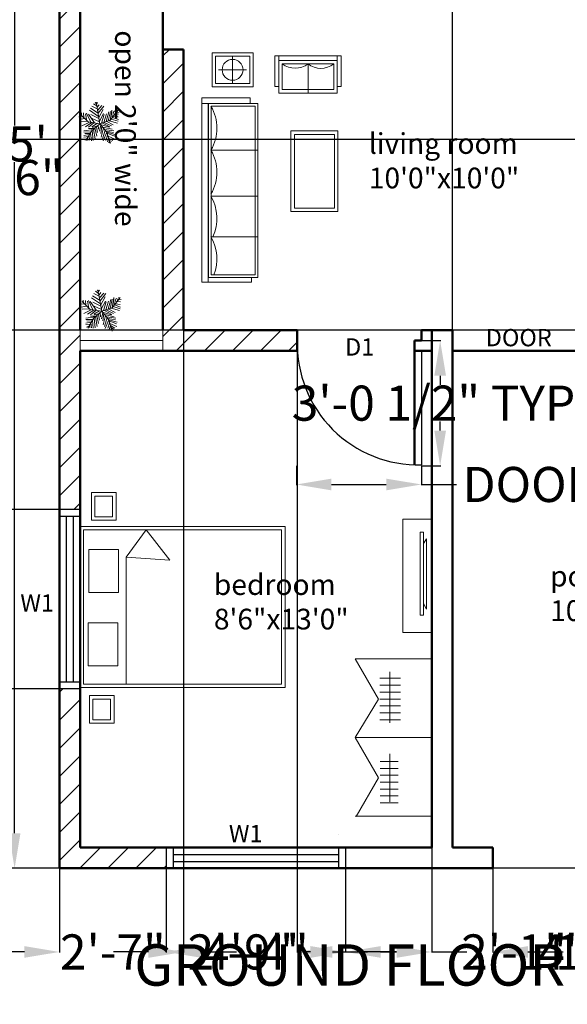
# Model space of a CAD drawing. Units: inches. Extents: x 21 to 3450, y 4 to 2137.
# Tile 9 of 14: x 2805 to 2964, y 1047 to 1333. Entities that reach past the tile are written whole.
import ezdxf

# ---------------------------------------------------------------- set-up
doc = ezdxf.new("R2010")
doc.units = ezdxf.units.IN
doc.header["$MEASUREMENT"] = 0
for name, color, linetype, lineweight in [('A-ANNO-DIMS', 2, 'Continuous', 18), ('A-ANNO-TEXT', 7, 'Continuous', 18), ('A-AREA-IDEN', 3, 'Continuous', 18), ('A-DOOR', 4, 'Continuous', 25), ('A-FURN', 8, 'Continuous', 18), ('A-GLAZ', 3, 'Continuous', 25), ('A-WALL', 7, 'Continuous', 50), ('A-WALL-PATT', 8, 'Continuous', 13), ('L-PLNT', 94, 'Continuous', 13)]:
    doc.layers.add(name, color=color, linetype=linetype, lineweight=lineweight)
doc.styles.get("Standard").update_dxf_attribs({"font": 'arial.ttf'})
doc.dimstyles.get("Standard").update_dxf_attribs({"dimtxt": 10.18, "dimasz": 10.18, "dimexe": 0.18, "dimexo": 0.0625, "dimgap": 0.09, "dimtad": 0, "dimtih": 1, "dimtoh": 1, "dimdec": 0, "dimzin": 0, "dimdsep": 46, "dimlunit": 3, "dimtxsty": 'Standard', "dimcen": 0.09, "dimadec": 0, "dimazin": 0, "dimtfac": 1, "dimtdec": 0, "dimtofl": 0, "dimtmove": 0, "dimatfit": 3, "dimfxl": 1, "dimtolj": 1, "dimtzin": 0, "dimarcsym": 0})

# ---------------------------------------------------------------- blocks, each defined once
blk = doc.blocks.new('*U6')
for p, q in [((-8.737, 47.138), (-17.069, 52.711)), ((-10.186, 53.64), (-13.084, 55.962)), ((0, 0), (-10.5, 57)), ((-9.099, 51.782), (-6.563, 55.962)), ((-48.585, 21.131), (-49.309, 29.026)), ((-43.513, 28.561), (-42.427, 15.558)), ((-38.442, 26.239), (-34.819, 7.663)), ((-35.544, 28.097), (-24.314, 3.947)), ((-3.665, 19.273), (-27.574, 35.527)), ((-5.114, 28.097), (-24.676, 40.636)), ((-7.288, 39.707), (-21.778, 46.673)), ((-7.65, 43.423), (-2.578, 49.46)), ((-5.839, 35.992), (4.667, 48.067)), ((-5.114, 27.632), (10.463, 46.673)), ((-2.941, 16.486), (8.652, 37.85)), ((-1.129, 6.734), (9.014, 26.704)), ((10.101, 3.483), (17.708, 26.239)), ((16.259, 5.805), (23.142, 31.348)), ((22.055, 7.198), (27.489, 32.277)), ((27, 9), (48, 36)), ((27.127, 9.056), (31.112, 35.992)), ((31.836, 30.883), (32.561, 16.486)), ((35.096, 32.741), (37.27, 22.524)), ((38.719, 34.134), (41.979, 28.561)), ((43.791, 29.954), (51.036, 30.883)), ((44.153, 36.456), (45.239, 32.741)), ((-47.498, 19.737), (-55.83, 18.344)), ((-40.615, 13.7), (-55.105, 10.913)), ((-31.5, 4.5), (-52.5, 25.5)), ((-33.37, 6.269), (-52.207, 5.34)), ((-28.299, 3.483), (-47.86, -5.805)), ((-21.416, 3.018), (-38.079, -8.128)), ((0, 0), (-31.5, 4.5)), ((-14.533, 2.09), (-30.834, 25.31)), ((-15.982, 2.09), (-30.11, -9.521)), ((-24.314, 23.917), (-2.941, 13.7)), ((0, 0), (-22.5, -19.5)), ((-6.563, 1.161), (-21.416, -8.128)), ((-20.691, 13.7), (-1.129, 4.876)), ((0, 0), (27, 9)), ((0, 0), (18, -22.5)), ((3.942, 1.625), (11.187, 24.381)), ((6.478, 1.625), (26.04, -8.592)), ((11.187, 3.483), (30.749, -5.805)), ((18.07, 5.805), (35.096, -3.483)), ((24.229, 7.663), (46.688, 1.625)), ((29.662, 12.307), (48.137, 6.269)), ((33.285, 16.486), (48.862, 10.913)), ((36.183, 19.737), (48.137, 17.88)), ((40.53, 25.775), (48.862, 24.846)), ((-17.431, -15.094), (-42.789, -18.809)), ((-24.314, -21.596), (-42.427, -22.06)), ((-26.849, -26.24), (-40.253, -25.775)), ((-22.5, -19.5), (-37.5, -45)), ((-15.257, -12.772), (-30.11, -12.772)), ((-25.038, -23.918), (-22.865, -45.281)), ((-20.691, -18.345), (-17.793, -44.352)), ((-6.563, -5.805), (-19.967, -9.985)), ((-17.069, -15.094), (-12.721, -40.172)), ((-13.446, -11.378), (-8.737, -32.741)), ((-9.461, -8.592), (-6.201, -23.453)), ((-4.752, -3.483), (-3.665, -14.629)), ((2.493, -3.019), (-1.491, -20.202)), ((1.769, -2.555), (24.229, -9.521)), ((5.029, -6.27), (2.131, -25.775)), ((9.014, -11.378), (3.58, -35.992)), ((14.085, -16.951), (6.478, -40.172)), ((7.565, -9.056), (32.198, -14.629)), ((18.07, -22.524), (8.289, -45.745)), ((12.274, -15.094), (36.907, -18.809)), ((16.259, -19.738), (36.183, -22.989)), ((18, -22.5), (27, -52.5)), ((18.433, -22.524), (40.53, -29.026)), ((19.157, -25.311), (38.719, -33.206)), ((-28.299, -29.026), (-42.789, -31.348)), ((-30.834, -34.135), (-42.427, -35.528)), ((-34.457, -39.708), (-40.978, -42.494)), ((-32.646, -36.921), (-31.921, -44.352)), ((-29.023, -30.884), (-27.936, -43.887)), ((20.244, -30.419), (15.897, -44.816)), ((22.78, -37.85), (19.519, -48.532)), ((21.331, -32.741), (39.081, -40.636)), ((22.78, -38.314), (34.372, -44.816)), ((24.591, -45.745), (23.142, -50.854)), ((24.591, -43.423), (30.749, -47.603)), ((26.764, -49.925), (28.213, -50.854))]:
    blk.add_line(p, q)
blk = doc.blocks.new('*D8')
at = {"layer": 'A-ANNO-DIMS', "color": 0, "lineweight": -2, "transparency": 16777216}
for p, q in [((2816.85, 1506.81), (2803.73, 1506.81)), ((2803.91, 1496.63), (2803.91, 1302.07)), ((2803.91, 1096.92), (2803.91, 1291.48)), ((2999.5, 1086.74), (2803.73, 1086.74))]:
    blk.add_line(p, q, dxfattribs=at)
at = {"layer": 'A-ANNO-DIMS', "color": 0, "transparency": 16777216}
for points in [[(2802.22, 1496.63), (2805.61, 1496.63), (2803.91, 1506.81)], [(2802.22, 1096.92), (2805.61, 1096.92), (2803.91, 1086.74)]]:
    blk.add_solid(points, dxfattribs=at)
at = {"layer": 'Defpoints', "color": 0, "transparency": 16777216}
for p in [(2816.91, 1506.81), (2803.91, 1086.74), (2999.56, 1086.74)]:
    blk.add_point(p, dxfattribs=at)
at = {"layer": 'A-ANNO-DIMS', "color": 0, "transparency": 16777216, "insert": (2803.91, 1296.77), "char_height": 10.18, "attachment_point": 5}
blk.add_mtext("\\A1;35'", dxfattribs=at)
blk = doc.blocks.new('DOOR-35IN')
blk.add_line((36, 33.01), (36, 0.01))
blk.add_arc((35, 35.01), 35.01, 178.3634, 271.6366)
blk = doc.blocks.new('SOFA-3SEAT')
blk.add_line((0, 36.17), (13.59, 36.17))
blk.add_lwpolyline([(0, 48.92), (12.82, 48.92), (12.82, 0), (0, 0)], close=True)
for centre in [(-11.01, 42.54), (-11.01, 29.79)]:
    blk.add_arc(centre, 12.72, 329.9119, 30.0881)
blk = doc.blocks.new('ARMCHAIR')
blk.add_line((7.48, 8.43), (7.48, 0))
blk.add_lwpolyline([(0, 8.43), (14.95, 8.43), (14.95, 1), (0, 1)], close=True)
for centre, radius, start, end in [((3.74, 13.52), 6.31, 233.6798, 306.3202), ((11.21, 13.17), 6.03, 231.7288, 308.2712)]:
    blk.add_arc(centre, radius, start, end)
blk = doc.blocks.new('*D26')
at = {"layer": 'A-ANNO-DIMS', "color": 0, "lineweight": -2, "transparency": 16777216}
for p, q in [((2885.64, 1203.41), (2885.64, 1197.85)), ((2921.91, 1203.41), (2921.91, 1197.85)), ((2895.82, 1198.03), (2911.73, 1198.03)), ((2921.91, 1198.03), (2932.09, 1198.03))]:
    blk.add_line(p, q, dxfattribs=at)
at = {"layer": 'A-ANNO-DIMS', "color": 0, "transparency": 16777216}
for points in [[(2895.82, 1199.72), (2895.82, 1196.33), (2885.64, 1198.03)], [(2911.73, 1199.72), (2911.73, 1196.33), (2921.91, 1198.03)]]:
    blk.add_solid(points, dxfattribs=at)
at = {"layer": 'Defpoints', "color": 0, "transparency": 16777216}
for p in [(2885.64, 1203.47), (2921.91, 1203.47), (2921.91, 1198.03)]:
    blk.add_point(p, dxfattribs=at)
at = {"layer": 'A-ANNO-DIMS', "color": 0, "transparency": 16777216, "insert": (3010.53, 1198.03), "char_height": 10.18, "attachment_point": 5}
blk.add_mtext('\\A1;DOOR 35" 3\'-0 1/2" TYP.', dxfattribs=at)
blk = doc.blocks.new('*D27')
at = {"layer": 'A-ANNO-DIMS', "color": 0, "lineweight": -2, "transparency": 16777216}
for p, q in [((2921.97, 1239.74), (2927.53, 1239.74)), ((2927.35, 1229.56), (2927.35, 1226.96)), ((2927.35, 1213.65), (2927.35, 1216.25)), ((2921.97, 1203.47), (2927.53, 1203.47))]:
    blk.add_line(p, q, dxfattribs=at)
at = {"layer": 'A-ANNO-DIMS', "color": 0, "transparency": 16777216}
for points in [[(2925.66, 1229.56), (2929.05, 1229.56), (2927.35, 1239.74)], [(2925.66, 1213.65), (2929.05, 1213.65), (2927.35, 1203.47)]]:
    blk.add_solid(points, dxfattribs=at)
at = {"layer": 'Defpoints', "color": 0, "transparency": 16777216}
for p in [(2921.91, 1239.74), (2927.35, 1239.74), (2921.91, 1203.47)]:
    blk.add_point(p, dxfattribs=at)
at = {"layer": 'A-ANNO-DIMS', "color": 0, "transparency": 16777216, "insert": (2927.35, 1221.61), "char_height": 10.18, "attachment_point": 5}
blk.add_mtext('\\A1;3\'-0 1/2" TYP.', dxfattribs=at)
blk = doc.blocks.new('*D77')
at = {"layer": 'A-ANNO-DIMS', "color": 0, "lineweight": -2, "transparency": 16777216}
for p, q in [((2778.96, 1276.83), (2778.96, 1287.01)), ((2778.96, 1287.01), (2789.14, 1287.01)), ((2749.77, 1266.65), (2779.14, 1266.65)), ((2749.77, 1260.65), (2779.14, 1260.65)), ((2778.96, 1250.47), (2778.96, 1240.29))]:
    blk.add_line(p, q, dxfattribs=at)
at = {"layer": 'A-ANNO-DIMS', "color": 0, "transparency": 16777216}
for points in [[(2777.26, 1276.83), (2780.65, 1276.83), (2778.96, 1266.65)], [(2777.26, 1250.47), (2780.65, 1250.47), (2778.96, 1260.65)]]:
    blk.add_solid(points, dxfattribs=at)
at = {"layer": 'Defpoints', "color": 0, "transparency": 16777216}
for p in [(2749.71, 1266.65), (2778.96, 1266.65), (2749.71, 1260.65)]:
    blk.add_point(p, dxfattribs=at)
at = {"layer": 'A-ANNO-DIMS', "color": 0, "transparency": 16777216, "insert": (2802.76, 1287.01), "char_height": 10.18, "attachment_point": 5}
blk.add_mtext('\\A1;0\'-6"', dxfattribs=at)
blk = doc.blocks.new('*D101')
at = {"layer": 'A-ANNO-DIMS', "color": 0, "lineweight": -2, "transparency": 16777216}
for p, q in [((2816.91, 1086.68), (2816.91, 1062.31)), ((2847.91, 1086.68), (2847.91, 1062.31)), ((2806.73, 1062.49), (2796.55, 1062.49)), ((2858.09, 1062.49), (2868.27, 1062.49))]:
    blk.add_line(p, q, dxfattribs=at)
at = {"layer": 'A-ANNO-DIMS', "color": 0, "transparency": 16777216}
for points in [[(2806.73, 1064.19), (2806.73, 1060.8), (2816.91, 1062.49)], [(2858.09, 1064.19), (2858.09, 1060.8), (2847.91, 1062.49)]]:
    blk.add_solid(points, dxfattribs=at)
at = {"layer": 'Defpoints', "color": 0, "transparency": 16777216}
for p in [(2816.91, 1086.74), (2847.91, 1086.74), (2847.91, 1062.49)]:
    blk.add_point(p, dxfattribs=at)
at = {"layer": 'A-ANNO-DIMS', "color": 0, "transparency": 16777216, "insert": (2832.41, 1062.49), "char_height": 10.18, "attachment_point": 5}
blk.add_mtext('\\A1;2\'-7"', dxfattribs=at)
blk = doc.blocks.new('*D102')
at = {"layer": 'A-ANNO-DIMS', "color": 0, "lineweight": -2, "transparency": 16777216}
for p, q in [((2847.91, 1086.68), (2847.91, 1062.31)), ((2899.91, 1086.68), (2899.91, 1062.31)), ((2858.09, 1062.49), (2860.09, 1062.49)), ((2889.73, 1062.49), (2887.74, 1062.49))]:
    blk.add_line(p, q, dxfattribs=at)
at = {"layer": 'A-ANNO-DIMS', "color": 0, "transparency": 16777216}
for points in [[(2858.09, 1064.19), (2858.09, 1060.8), (2847.91, 1062.49)], [(2889.73, 1064.19), (2889.73, 1060.8), (2899.91, 1062.49)]]:
    blk.add_solid(points, dxfattribs=at)
at = {"layer": 'Defpoints', "color": 0, "transparency": 16777216}
for p in [(2847.91, 1086.74), (2899.91, 1086.74), (2899.91, 1062.49)]:
    blk.add_point(p, dxfattribs=at)
at = {"layer": 'A-ANNO-DIMS', "color": 0, "transparency": 16777216, "insert": (2873.91, 1062.49), "char_height": 10.18, "attachment_point": 5}
blk.add_mtext('\\A1;4\'-4"', dxfattribs=at)
blk = doc.blocks.new('*D103')
at = {"layer": 'A-ANNO-DIMS', "color": 0, "lineweight": -2, "transparency": 16777216}
for p, q in [((2924.91, 1092.68), (2924.91, 1062.31)), ((2899.91, 1086.68), (2899.91, 1062.31)), ((2910.09, 1062.49), (2914.73, 1062.49)), ((2924.91, 1062.49), (2935.09, 1062.49))]:
    blk.add_line(p, q, dxfattribs=at)
at = {"layer": 'A-ANNO-DIMS', "color": 0, "transparency": 16777216}
for points in [[(2910.09, 1064.19), (2910.09, 1060.8), (2899.91, 1062.49)], [(2914.73, 1064.19), (2914.73, 1060.8), (2924.91, 1062.49)]]:
    blk.add_solid(points, dxfattribs=at)
at = {"layer": 'Defpoints', "color": 0, "transparency": 16777216}
for p in [(2924.91, 1092.74), (2899.91, 1086.74), (2924.91, 1062.49)]:
    blk.add_point(p, dxfattribs=at)
at = {"layer": 'A-ANNO-DIMS', "color": 0, "transparency": 16777216, "insert": (2948.8, 1062.49), "char_height": 10.18, "attachment_point": 5}
blk.add_mtext('\\A1;2\'-1"', dxfattribs=at)
blk = doc.blocks.new('*D104')
at = {"layer": 'A-ANNO-DIMS', "color": 0, "lineweight": -2, "transparency": 16777216}
for p, q in [((2924.91, 1092.68), (2924.91, 1062.31)), ((2942.64, 1086.68), (2942.64, 1062.31)), ((2914.73, 1062.49), (2904.55, 1062.49)), ((2952.82, 1062.49), (2963, 1062.49))]:
    blk.add_line(p, q, dxfattribs=at)
at = {"layer": 'A-ANNO-DIMS', "color": 0, "transparency": 16777216}
for points in [[(2914.73, 1064.19), (2914.73, 1060.8), (2924.91, 1062.49)], [(2952.82, 1064.19), (2952.82, 1060.8), (2942.64, 1062.49)]]:
    blk.add_solid(points, dxfattribs=at)
at = {"layer": 'Defpoints', "color": 0, "transparency": 16777216}
for p in [(2924.91, 1092.74), (2942.64, 1086.74), (2942.64, 1062.49)]:
    blk.add_point(p, dxfattribs=at)
at = {"layer": 'A-ANNO-DIMS', "color": 0, "transparency": 16777216, "insert": (2988, 1062.49), "char_height": 10.18, "attachment_point": 5}
blk.add_mtext('\\A1;1\'-5 1/2"', dxfattribs=at)
blk = doc.blocks.new('*D105')
at = {"layer": 'A-ANNO-DIMS', "color": 0, "lineweight": -2, "transparency": 16777216}
for p, q in [((2942.64, 1086.68), (2942.64, 1062.31)), ((2999.56, 1086.68), (2999.56, 1062.31)), ((2952.82, 1062.49), (2957.27, 1062.49)), ((2989.38, 1062.49), (2984.92, 1062.49))]:
    blk.add_line(p, q, dxfattribs=at)
at = {"layer": 'A-ANNO-DIMS', "color": 0, "transparency": 16777216}
for points in [[(2952.82, 1064.19), (2952.82, 1060.8), (2942.64, 1062.49)], [(2989.38, 1064.19), (2989.38, 1060.8), (2999.56, 1062.49)]]:
    blk.add_solid(points, dxfattribs=at)
at = {"layer": 'Defpoints', "color": 0, "transparency": 16777216}
for p in [(2942.64, 1086.74), (2999.56, 1086.74), (2999.56, 1062.49)]:
    blk.add_point(p, dxfattribs=at)
at = {"layer": 'A-ANNO-DIMS', "color": 0, "transparency": 16777216, "insert": (2971.1, 1062.49), "char_height": 10.18, "attachment_point": 5}
blk.add_mtext('\\A1;4\'-9"', dxfattribs=at)
blk = doc.blocks.new('*D114')
at = {"layer": 'A-ANNO-DIMS', "color": 0, "lineweight": -2, "transparency": 16777216}
for p, q in [((2816.85, 1138.74), (2738.48, 1138.74)), ((2738.66, 1128.56), (2738.66, 1117.92)), ((2738.66, 1096.92), (2738.66, 1107.56)), ((2816.85, 1086.74), (2738.48, 1086.74))]:
    blk.add_line(p, q, dxfattribs=at)
at = {"layer": 'A-ANNO-DIMS', "color": 0, "transparency": 16777216}
for points in [[(2736.97, 1128.56), (2740.36, 1128.56), (2738.66, 1138.74)], [(2736.97, 1096.92), (2740.36, 1096.92), (2738.66, 1086.74)]]:
    blk.add_solid(points, dxfattribs=at)
at = {"layer": 'Defpoints', "color": 0, "transparency": 16777216}
for p in [(2738.66, 1138.74), (2816.91, 1138.74), (2816.91, 1086.74)]:
    blk.add_point(p, dxfattribs=at)
at = {"layer": 'A-ANNO-DIMS', "color": 0, "transparency": 16777216, "insert": (2738.66, 1112.74), "char_height": 10.18, "attachment_point": 5}
blk.add_mtext('\\A1;4\'-4"', dxfattribs=at)
blk = doc.blocks.new('*D115')
at = {"layer": 'A-ANNO-DIMS', "color": 0, "lineweight": -2, "transparency": 16777216}
for p, q in [((2816.85, 1190.74), (2738.48, 1190.74)), ((2738.66, 1180.56), (2738.66, 1169.92)), ((2738.66, 1148.92), (2738.66, 1159.56)), ((2816.85, 1138.74), (2738.48, 1138.74))]:
    blk.add_line(p, q, dxfattribs=at)
at = {"layer": 'A-ANNO-DIMS', "color": 0, "transparency": 16777216}
for points in [[(2736.97, 1180.56), (2740.36, 1180.56), (2738.66, 1190.74)], [(2736.97, 1148.92), (2740.36, 1148.92), (2738.66, 1138.74)]]:
    blk.add_solid(points, dxfattribs=at)
at = {"layer": 'Defpoints', "color": 0, "transparency": 16777216}
for p in [(2738.66, 1190.74), (2816.91, 1190.74), (2816.91, 1138.74)]:
    blk.add_point(p, dxfattribs=at)
at = {"layer": 'A-ANNO-DIMS', "color": 0, "transparency": 16777216, "insert": (2738.66, 1164.74), "char_height": 10.18, "attachment_point": 5}
blk.add_mtext('\\A1;4\'-4"', dxfattribs=at)
blk = doc.blocks.new('*D117')
at = {"layer": 'A-ANNO-DIMS', "color": 0, "lineweight": -2, "transparency": 16777216}
for p, q in [((2852.91, 1242.68), (2852.91, 1062.31)), ((2885.91, 1242.68), (2885.91, 1062.31)), ((2842.73, 1062.49), (2832.55, 1062.49)), ((2896.09, 1062.49), (2906.27, 1062.49))]:
    blk.add_line(p, q, dxfattribs=at)
at = {"layer": 'A-ANNO-DIMS', "color": 0, "transparency": 16777216}
for points in [[(2842.73, 1064.19), (2842.73, 1060.8), (2852.91, 1062.49)], [(2896.09, 1064.19), (2896.09, 1060.8), (2885.91, 1062.49)]]:
    blk.add_solid(points, dxfattribs=at)
at = {"layer": 'Defpoints', "color": 0, "transparency": 16777216}
for p in [(2852.91, 1242.74), (2885.91, 1242.74), (2885.91, 1062.49)]:
    blk.add_point(p, dxfattribs=at)
at = {"layer": 'A-ANNO-DIMS', "color": 0, "transparency": 16777216, "insert": (2869.41, 1062.49), "char_height": 10.18, "attachment_point": 5}
blk.add_mtext('\\A1;2\'-9"', dxfattribs=at)
blk = doc.blocks.new('*D118')
at = {"layer": 'A-ANNO-DIMS', "color": 0, "lineweight": -2, "transparency": 16777216}
for p, q in [((2920.73, 1539.16), (2910.55, 1539.16)), ((2930.91, 1242.81), (2930.91, 1539.34)), ((2972.91, 1242.81), (2972.91, 1539.34)), ((2983.09, 1539.16), (2993.27, 1539.16))]:
    blk.add_line(p, q, dxfattribs=at)
at = {"layer": 'A-ANNO-DIMS', "color": 0, "transparency": 16777216}
for points in [[(2920.73, 1540.85), (2920.73, 1537.46), (2930.91, 1539.16)], [(2983.09, 1540.85), (2983.09, 1537.46), (2972.91, 1539.16)]]:
    blk.add_solid(points, dxfattribs=at)
at = {"layer": 'Defpoints', "color": 0, "transparency": 16777216}
for p in [(2972.91, 1539.16), (2930.91, 1242.74), (2972.91, 1242.74)]:
    blk.add_point(p, dxfattribs=at)
at = {"layer": 'A-ANNO-DIMS', "color": 0, "transparency": 16777216, "insert": (2951.91, 1539.16), "char_height": 10.18, "attachment_point": 5}
blk.add_mtext('\\A1;3\'-6"', dxfattribs=at)
blk = doc.blocks.new('*D120')
at = {"layer": 'A-ANNO-DIMS', "color": 0, "lineweight": -2, "transparency": 16777216}
for p, q in [((2972.85, 1298.07), (2738.48, 1298.07)), ((2738.66, 1287.89), (2738.66, 1275.76)), ((2738.66, 1252.92), (2738.66, 1265.05)), ((2972.85, 1242.74), (2738.48, 1242.74))]:
    blk.add_line(p, q, dxfattribs=at)
at = {"layer": 'A-ANNO-DIMS', "color": 0, "transparency": 16777216}
for points in [[(2736.97, 1287.89), (2740.36, 1287.89), (2738.66, 1298.07)], [(2736.97, 1252.92), (2740.36, 1252.92), (2738.66, 1242.74)]]:
    blk.add_solid(points, dxfattribs=at)
at = {"layer": 'Defpoints', "color": 0, "transparency": 16777216}
for p in [(2738.66, 1298.07), (2972.91, 1298.07), (2972.91, 1242.74)]:
    blk.add_point(p, dxfattribs=at)
at = {"layer": 'A-ANNO-DIMS', "color": 0, "transparency": 16777216, "insert": (2738.66, 1270.41), "char_height": 10.18, "attachment_point": 5}
blk.add_mtext('\\A1;4\'-7 1/2"', dxfattribs=at)

msp = doc.modelspace()

# ---------------------------------------------------------------- hatches: boundary and pattern name
at = {"layer": 'A-WALL-PATT'}
h = msp.add_hatch(dxfattribs=at)
h.set_pattern_fill('ANSI31', color=256, scale=46)
h.set_pattern_definition([(45, (-32.016, 151.0237), (-4.065864, 4.065864), [])])
h.paths.add_polyline_path([(2951.41, 1506.74), (2816.91, 1506.74), (2816.91, 1190.74), (2822.91, 1190.74), (2822.91, 1236.74), (2822.91, 1242.74), (2822.91, 1362.74), (2822.91, 1368.74), (2822.91, 1452.74), (2846.41, 1452.74), (2846.41, 1458.74), (2822.91, 1458.74), (2822.91, 1500.74), (2897.91, 1500.74), (2903.91, 1500.74), (2951.41, 1500.74)])
h.paths.add_polyline_path([(3056.91, 1506.74), (3003.41, 1506.74), (3003.41, 1500.74), (3050.91, 1500.74), (3050.91, 1460.31, -0.065004), (3051.05, 1459.28), (3051.05, 1422.47, -0.065004), (3050.91, 1421.45), (3050.91, 1368.74), (2942.4, 1368.74), (2942.4, 1365.74), (2944.4, 1365.74), (2944.4, 1362.74), (2972.91, 1362.74), (2972.91, 1336.29), (2978.91, 1336.29), (2978.91, 1362.74), (3050.91, 1362.74), (3050.91, 1328.74), (3056.91, 1328.74)])
h.paths.add_polyline_path([(2885.91, 1239.74), (2885.91, 1242.74), (2852.91, 1242.74), (2852.91, 1324.17), (2846.91, 1324.17), (2846.91, 1242.74), (2846.91, 1236.74), (2885.91, 1236.74), (2885.91, 1237.74, -0.014283)], flags=17)
h.paths.add_polyline_path([(2847.91, 1092.74), (2822.91, 1092.74), (2822.91, 1138.74), (2816.91, 1138.74), (2816.91, 1086.74), (2847.91, 1086.74)])
h.paths.add_polyline_path([(2911.4, 1368.74), (2903.91, 1368.74), (2897.91, 1368.74), (2846.91, 1368.74), (2846.91, 1362.74), (2852.91, 1362.74), (2903.91, 1362.74), (2911.4, 1362.74)], flags=17)
h.paths.add_polyline_path([(2903.91, 1458.74), (2897.91, 1458.74), (2874.41, 1458.74), (2874.41, 1452.74), (2897.91, 1452.74), (2897.91, 1401.74), (2898.91, 1401.74, -0.017236), (2900.91, 1401.74), (2903.91, 1401.74), (2903.91, 1452.74)], flags=17)

# ---------------------------------------------------------------- linework, layer by layer
at = {"layer": 'A-FURN'}
for p, q in [((2867.14, 1322.19), (2867.14, 1314.33)), ((2863.02, 1318.26), (2871.19, 1318.27)), ((2860.88, 1281.6), (2874.47, 1281.6)), ((2860.88, 1269.84), (2874.47, 1269.84)), ((2860.06, 1256.66), (2858.21, 1256.66)), ((2822.91, 1242.74), (2846.91, 1242.74)), ((2822.91, 1242.74), (2822.91, 1236.74)), ((2846.91, 1242.74), (2846.91, 1236.74)), ((2846.91, 1239.74), (2822.91, 1239.74)), ((2836.24, 1176.98), (2842.11, 1184.86)), ((2842.11, 1184.86), (2848.89, 1176.12)), ((2922.52, 1180.94), (2923.37, 1182.26)), ((2923.37, 1182.26), (2923.37, 1161.86)), ((2836.24, 1140.16), (2836.24, 1176.98)), ((2848.89, 1176.12), (2836.24, 1176.98)), ((2923.37, 1161.86), (2922.52, 1163.56)), ((2902.74, 1147.44), (2909.45, 1135.81)), ((2912.79, 1143.72), (2912.79, 1128.88)), ((2909.89, 1141.83), (2915.8, 1141.83)), ((2909.89, 1139.83), (2915.8, 1139.83)), ((2909.89, 1137.83), (2915.8, 1137.83)), ((2909.45, 1135.81), (2902.74, 1124.65)), ((2909.89, 1135.83), (2915.8, 1135.83)), ((2909.89, 1133.83), (2915.8, 1133.83)), ((2909.89, 1131.83), (2915.8, 1131.83)), ((2909.89, 1129.83), (2915.8, 1129.83)), ((2902.74, 1124.65), (2924.91, 1124.65)), ((2902.74, 1124.65), (2909.47, 1112.99)), ((2912.79, 1119.91), (2912.79, 1105.99)), ((2909.93, 1117.71), (2915.15, 1117.71)), ((2909.93, 1115.71), (2915.15, 1115.71)), ((2909.93, 1113.71), (2915.15, 1113.71)), ((2909.47, 1112.99), (2902.97, 1101.73)), ((2909.93, 1111.71), (2915.15, 1111.71)), ((2909.93, 1109.71), (2915.15, 1109.71)), ((2909.93, 1107.71), (2915.15, 1107.71)), ((2909.93, 1105.71), (2915.15, 1105.71))]:
    msp.add_line(p, q, dxfattribs=at)
for points in [[(2861.17, 1323.19), (2873.11, 1323.19), (2873.11, 1313.33), (2861.17, 1313.33)], [(2862.17, 1322.19), (2862.17, 1322.19), (2872.11, 1322.19), (2872.11, 1322.19), (2872.11, 1314.33), (2872.11, 1314.33), (2862.17, 1314.33), (2862.17, 1314.33)], [(2880.54, 1313.45), (2880.54, 1313.45), (2879.36, 1313.45), (2879.36, 1313.45), (2879.36, 1322.33), (2879.36, 1322.33), (2880.54, 1322.33), (2880.54, 1322.33)], [(2880.54, 1322.33), (2880.54, 1322.33), (2897.49, 1322.33), (2897.49, 1322.33), (2897.49, 1320.95), (2897.49, 1320.95), (2880.54, 1320.95), (2880.54, 1320.95)], [(2898.67, 1313.45), (2898.67, 1313.45), (2897.49, 1313.45), (2897.49, 1313.45), (2897.49, 1322.33), (2897.49, 1322.33), (2898.67, 1322.33), (2898.67, 1322.33)], [(2880.54, 1320.95), (2880.54, 1320.95), (2897.49, 1320.95), (2897.49, 1320.95), (2897.49, 1311.52), (2897.49, 1311.52), (2880.54, 1311.52), (2880.54, 1311.52)], [(2872.25, 1308.48), (2872.25, 1308.48), (2858.21, 1308.48), (2858.21, 1308.48), (2858.21, 1310.12), (2858.21, 1310.12), (2872.25, 1310.12), (2872.25, 1310.12)], [(2860.12, 1308.48), (2860.12, 1308.48), (2874.47, 1308.48), (2874.47, 1308.48), (2874.47, 1258.03), (2874.47, 1258.03), (2860.12, 1258.03), (2860.12, 1258.03)], [(2884.06, 1300.54), (2884.06, 1300.54), (2897.68, 1300.54), (2897.68, 1300.54), (2897.68, 1277.18), (2897.68, 1277.18), (2884.06, 1277.18), (2884.06, 1277.18)], [(2885.06, 1299.54), (2896.68, 1299.54), (2896.68, 1278.18), (2885.06, 1278.18)], [(2860.06, 1258.03), (2860.06, 1258.03), (2872.59, 1258.03), (2872.59, 1258.03), (2872.59, 1256.66), (2872.59, 1256.66), (2860.06, 1256.66), (2860.06, 1256.66)], [(2826.2, 1195.67), (2826.2, 1195.67), (2833.35, 1195.67), (2833.35, 1195.67), (2833.35, 1187.69), (2833.35, 1187.69), (2826.2, 1187.69), (2826.2, 1187.69)], [(2827.2, 1194.67), (2832.35, 1194.67), (2832.35, 1188.69), (2827.2, 1188.69)], [(2924.91, 1188.02), (2924.91, 1188.02), (2916.52, 1188.02), (2916.52, 1188.02), (2916.52, 1155.13), (2916.52, 1155.13), (2924.91, 1155.13), (2924.91, 1155.13)], [(2822.91, 1185.86), (2822.91, 1185.86), (2882.37, 1185.86), (2882.37, 1185.86), (2882.37, 1139.16), (2882.37, 1139.16), (2822.91, 1139.16), (2822.91, 1139.16)], [(2823.91, 1184.86), (2881.37, 1184.86), (2881.37, 1140.16), (2823.91, 1140.16)], [(2921.56, 1184.2), (2921.56, 1184.2), (2922.52, 1184.2), (2922.52, 1184.2), (2922.52, 1160.1), (2922.52, 1160.1), (2921.56, 1160.1), (2921.56, 1160.1)], [(2825.47, 1179.17), (2825.47, 1179.17), (2834.06, 1179.17), (2834.06, 1179.17), (2834.06, 1166.72), (2834.06, 1166.72), (2825.47, 1166.72), (2825.47, 1166.72)], [(2825.27, 1157.88), (2825.27, 1157.88), (2833.86, 1157.88), (2833.86, 1157.88), (2833.86, 1145.42), (2833.86, 1145.42), (2825.27, 1145.42), (2825.27, 1145.42)], [(2825.6, 1136.82), (2825.6, 1136.82), (2832.75, 1136.82), (2832.75, 1136.82), (2832.75, 1128.84), (2832.75, 1128.84), (2825.6, 1128.84), (2825.6, 1128.84)], [(2826.6, 1135.82), (2831.75, 1135.82), (2831.75, 1129.84), (2826.6, 1129.84)]]:
    msp.add_lwpolyline(points, close=True, dxfattribs=at)
for points in [[(2858.21, 1256.66), (2858.21, 1308.48), (2858.21, 1308.48), (2860.06, 1308.48), (2860.06, 1308.48), (2860.06, 1256.66)], [(2902.74, 1101.86), (2902.74, 1101.86), (2924.91, 1101.86), (2924.91, 1101.86), (2924.91, 1147.44), (2924.91, 1147.44), (2902.74, 1147.44), (2902.74, 1147.44)]]:
    msp.add_lwpolyline(points, dxfattribs=at)
msp.add_circle((2867.14, 1318.26), 3.03, dxfattribs=at)
for centre, start, end in [((2849.87, 1301.34), 323.186, 323.6288), ((2849.87, 1275.22), 334.9772, 30.0881), ((2849.87, 1263.46), 338.4844, 30.0881)]:
    msp.add_arc(centre, 12.72, start, end, dxfattribs=at)
at = {"layer": 'A-GLAZ'}
for p, q in [((2822.91, 1190.74), (2816.91, 1190.74)), ((2822.91, 1188.74), (2816.91, 1188.74)), ((2818.91, 1188.74), (2818.91, 1140.74)), ((2820.91, 1188.74), (2820.91, 1140.74)), ((2822.91, 1140.74), (2816.91, 1140.74)), ((2822.91, 1138.74), (2816.91, 1138.74)), ((2847.91, 1092.74), (2847.91, 1086.74)), ((2849.91, 1092.74), (2849.91, 1086.74)), ((2849.91, 1090.74), (2897.91, 1090.74)), ((2897.91, 1092.74), (2897.91, 1086.74)), ((2899.91, 1092.74), (2899.91, 1086.74)), ((2849.91, 1088.74), (2897.91, 1088.74))]:
    msp.add_line(p, q, dxfattribs=at)
msp.add_lwpolyline([(2897.77, 1096.6), (2897.77, 1096.6)], close=True, dxfattribs=at)
at = {"layer": 'A-WALL'}
for p, q in [((2816.91, 1086.74), (2816.91, 1506.74)), ((2822.91, 1242.74), (2822.91, 1362.74)), ((2846.91, 1362.74), (2846.91, 1242.74)), ((2846.91, 1324.17), (2852.91, 1324.17)), ((2852.91, 1324.17), (2852.91, 1242.74)), ((2852.91, 1242.74), (2885.91, 1242.74)), ((2885.91, 1236.74), (2885.91, 1242.74)), ((2921.91, 1242.74), (2930.91, 1242.74)), ((2921.91, 1239.74), (2921.91, 1242.74)), ((2924.91, 1236.74), (2924.91, 1242.74)), ((2930.91, 1236.74), (2930.91, 1242.74)), ((2919.91, 1239.74), (2919.91, 1203.74)), ((2919.91, 1239.74), (2921.91, 1239.74)), ((2822.91, 1092.74), (2822.91, 1236.74)), ((2822.91, 1236.74), (2885.95, 1236.74)), ((2919.91, 1236.74), (2924.91, 1236.74)), ((2924.91, 1092.74), (2924.91, 1236.74)), ((2930.91, 1092.74), (2930.91, 1236.74)), ((2930.91, 1236.74), (3050.91, 1236.74)), ((2924.91, 1092.74), (2822.91, 1092.74)), ((2942.64, 1092.74), (2930.91, 1092.74)), ((2942.64, 1092.74), (2942.64, 1086.74)), ((2942.64, 1086.74), (2816.91, 1086.74))]:
    msp.add_line(p, q, dxfattribs=at)

# ---------------------------------------------------------------- block references
at = {"layer": 'A-DOOR'}
msp.add_blockref('DOOR-35IN', (2885.91, 1203.74), dxfattribs=at)
at = {"layer": 'A-FURN'}
for name, p in [('ARMCHAIR', (2881.54, 1311.52)), ('SOFA-3SEAT', (2860.88, 1258.8))]:
    msp.add_blockref(name, p, dxfattribs=at)
at = {"layer": 'L-PLNT', "xscale": 0.1095009231923873, "yscale": 0.1095009231923873, "zscale": 0.1095009231923873}
for p in [(2828.67, 1302.64), (2829.24, 1248.27)]:
    msp.add_blockref('*U6', p, dxfattribs=at)

# ---------------------------------------------------------------- texts
at = {"layer": 'A-ANNO-TEXT', "insert": (2839.06, 1329.7), "char_height": 6, "attachment_point": 1, "rotation": 270}
msp.add_mtext_dynamic_manual_height_columns('open 2\'0" wide', width=84.0083, gutter_width=1, heights=[0], dxfattribs=at)
at = {"layer": 'A-ANNO-TEXT', "attachment_point": 1}
for s, width, insert, char_height in [('DOOR', 14.628, (2940.58, 1243.1), 5), ('D1', 14.628, (2899.77, 1240.4), 5), ('W1', 14.628, (2805.56, 1166.19), 5), ('W1', 14.628, (2866.06, 1099.32), 5), ('GROUND FLOOR PLAN', 189.6067, (2838.61, 1064.72), 12)]:
    msp.add_mtext_dynamic_manual_height_columns(s, width=width, gutter_width=1, heights=[0], dxfattribs=dict(at, insert=insert, char_height=char_height))
at = {"layer": 'A-AREA-IDEN', "char_height": 6, "attachment_point": 1}
for s, insert in [('living room\\P10\'0"x10\'0"', (2906.65, 1299.89)), ('porch\\P10\'0"x13\'0"', (2959.24, 1174.45)), ('bedroom\\P8\'6"x13\'0"', (2861.71, 1172))]:
    msp.add_mtext_dynamic_manual_height_columns(s, width=84.0083, gutter_width=1, heights=[0], dxfattribs=dict(at, insert=insert))

# ---------------------------------------------------------------- dimensions: what is measured, and where the dimension line sits
at = {"layer": 'A-ANNO-DIMS'}
for base, p1, p2, picture, middle in [((2972.91, 1539.16), (2930.91, 1242.74), (2972.91, 1242.74), '*D118', (2951.91, 1539.16)), ((2885.91, 1062.49), (2852.91, 1242.74), (2885.91, 1242.74), '*D117', (2869.41, 1062.49)), ((2924.91, 1062.49), (2899.91, 1086.74), (2924.91, 1092.74), '*D103', (2948.8, 1062.49)), ((2942.64, 1062.49), (2924.91, 1092.74), (2942.64, 1086.74), '*D104', (2988, 1062.49)), ((2847.91, 1062.49), (2816.91, 1086.74), (2847.91, 1086.74), '*D101', (2832.41, 1062.49)), ((2899.91, 1062.49), (2847.91, 1086.74), (2899.91, 1086.74), '*D102', (2873.91, 1062.49)), ((2999.56, 1062.49), (2942.64, 1086.74), (2999.56, 1086.74), '*D105', (2971.1, 1062.49))]:
    dim = msp.add_linear_dim(base=base, p1=p1, p2=p2, dimstyle='Standard', override={"dimdec": 1, "dimlfac": 1, "dimrnd": 0, "dimzin": 1, "dimdsep": 46, "dimlunit": 4, "dimfrac": 2}, dxfattribs=at)
    dim.commit()
    dim.dimension.update_dxf_attribs({"geometry": picture, "text_midpoint": middle})
for base, p1, p2, override, picture, middle in [((2803.91, 1086.74), (2816.91, 1506.81), (2999.56, 1086.74), {"dimclrd": 0, "dimclre": 0, "dimclrt": 0}, '*D8', (2803.91, 1296.77)), ((2738.66, 1298.07), (2972.91, 1242.74), (2972.91, 1298.07), {"dimdec": 1, "dimlfac": 1, "dimrnd": 0, "dimzin": 1, "dimdsep": 46, "dimlunit": 4, "dimfrac": 2}, '*D120', (2738.66, 1270.41)), ((2778.96, 1266.65), (2749.71, 1260.65), (2749.71, 1266.65), {"dimdec": 1, "dimlfac": 1, "dimrnd": 0, "dimzin": 1, "dimdsep": 46, "dimlunit": 4, "dimfrac": 2}, '*D77', (2802.76, 1287.01)), ((2738.66, 1190.74), (2816.91, 1138.74), (2816.91, 1190.74), {"dimdec": 1, "dimlfac": 1, "dimrnd": 0, "dimzin": 1, "dimdsep": 46, "dimlunit": 4, "dimfrac": 2}, '*D115', (2738.66, 1164.74)), ((2738.66, 1138.74), (2816.91, 1086.74), (2816.91, 1138.74), {"dimdec": 1, "dimlfac": 1, "dimrnd": 0, "dimzin": 1, "dimdsep": 46, "dimlunit": 4, "dimfrac": 2}, '*D114', (2738.66, 1112.74))]:
    dim = msp.add_linear_dim(base=base, p1=p1, p2=p2, angle=90, dimstyle='Standard', override=override, dxfattribs=at)
    dim.commit()
    dim.dimension.update_dxf_attribs({"geometry": picture, "text_midpoint": middle})
dim = msp.add_linear_dim(base=(2927.35, 1239.74), p1=(2921.91, 1203.47), p2=(2921.91, 1239.74), angle=90, text='<> TYP.', dimstyle='Standard', override={"dimdec": 1, "dimrnd": 0, "dimzin": 1, "dimlunit": 4, "dimfrac": 2}, dxfattribs=at)
dim.commit()
dim.dimension.update_dxf_attribs({"geometry": '*D27', "text_midpoint": (2927.35, 1221.61)})
dim = msp.add_linear_dim(base=(2921.91, 1198.03), p1=(2885.64, 1203.47), p2=(2921.91, 1203.47), text='DOOR 35" <> TYP.', dimstyle='Standard', override={"dimdec": 1, "dimrnd": 0, "dimzin": 1, "dimlunit": 4, "dimfrac": 2}, dxfattribs=at)
dim.commit()
dim.dimension.update_dxf_attribs({"geometry": '*D26', "text_midpoint": (3010.53, 1198.03)})

doc.saveas('drawing.dxf')
